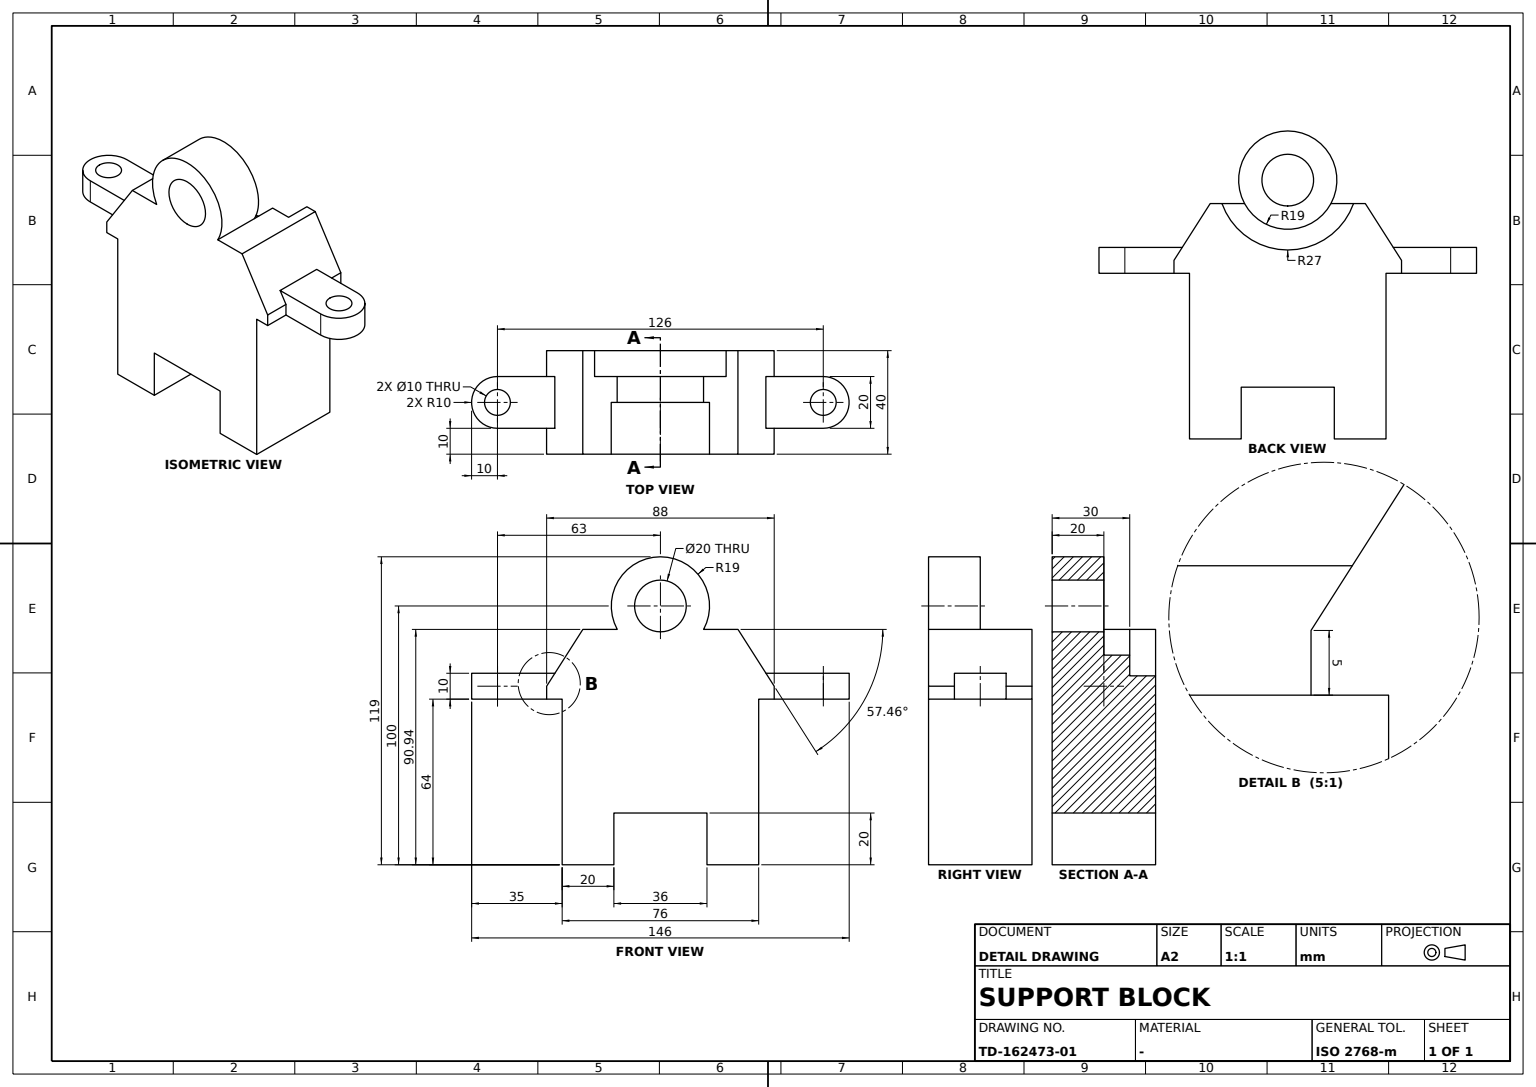
CATIA V5 part; units mm, degrees
sketch "Sketch1" plane through (0, 0, 0) normal (0, 1, 0) x (-1, 0, 0)
  point P0 (-38, 0)
  line L0 (-38, 0) -> (-18, 0)
  line L1 (38, 0) -> (38, 64)
  line L2 (-38, 64) -> (-38, 0)
  line L3 (-38, 64) -> (-44, 64)
  line L4 (-44, 64) -> (-44, 69)
  line L5 (44, 69) -> (44, 64)
  line L6 (44, 64) -> (38, 64)
  line L7 (-18, 0) -> (-18, 20)
  line L8 (-18, 20) -> (18, 20)
  line L9 (18, 20) -> (18, 0)
  point P1 (18, 0)
  line L10 (18, 0) -> (38, 0)
  arc A0 (-25.4361, 90.9444) -> (25.4361, 90.9444) centre (0, 100) ccw
  point P2 (0, 100)
  line L11 (-44, 69) -> (-30, 90.9444)
  point P3 (-30, 90.9444)
  line L12 (44, 69) -> (30, 90.9444)
  point P4 (30, 90.9444)
  line L13 (-30, 90.9444) -> (-25.4361, 90.9444)
  line L14 (25.4361, 90.9444) -> (30, 90.9444)
  dimension "length L1" = 64
  dimension "length L2" = 64
  dimension "distance L2 L1" = 76
  dimension "length L8" = 36
  dimension "length L9" = 20
  dimension "length L5" = 5
  dimension "length L4" = 5
  dimension "distance L4 L5" = 88
  dimension "radius A0" = 27
  dimension "distance P2 L6" = 36
  dimension "distance P2 y axis" = 0
  dimension "distance P3 P4" = 60
  constraint coincidence P0 x-axis
  constraint coincidence P1 L0
  constraint coincidence L0 L10
  constraint horizontal L0 x-axis
  constraint horizontal L3 x-axis
  constraint horizontal L6 x-axis
  constraint horizontal L8 x-axis
  constraint horizontal L10 x-axis
  constraint horizontal L13 x-axis
  constraint horizontal L14 x-axis
  constraint vertical L1 y-axis
  constraint vertical L2 y-axis
  constraint vertical L4 y-axis
  constraint vertical L5 y-axis
  constraint vertical L7 y-axis
  constraint vertical L9 y-axis
  constraint symmetry L2 L1 y-axis
  constraint symmetry L4 L5 y-axis
  constraint symmetry L7 L9 y-axis
  constraint symmetry P3 P4 y-axis
extrude "Pad1" add sketch "Sketch1" along normal mid plane 40
sketch "Sketch2" plane through (0, -20, 0) normal (0, -1, 0) x (1, 0, 0)
  arc A0 (-25.4361, 90.9444) -> (25.4361, 90.9444) centre (0, 100) ccw
  arc A1 (-16.7032, 90.9444) -> (16.7032, 90.9444) centre (0, 100) ccw
  point P0 (0, 100)
  line L0 (-25.4361, 90.9444) -> (-16.7032, 90.9444)
  point P1 (16.7032, 90.9444)
  line L1 (16.7032, 90.9444) -> (25.4361, 90.9444)
  point P2 (11.4413, 84.831)
  dimension "radius A1" = 19
  constraint coincidence P0 y-axis
  constraint coincidence L0 P1
  constraint coincidence L0 L1
  constraint coincidence P2 A1
  constraint concentricity A1 A0
  constraint horizontal L0 x-axis
  constraint horizontal L1 x-axis
extrude "Pad2" add sketch "Sketch2" against normal blind 30
sketch "Sketch3" plane through (0, -20, 0) normal (0, -1, 0) x (1, 0, 0)
  circle A0 centre (0, 100) radius 19
  point P0 (0, 100)
  arc A1 (-16.7032, 90.9444) -> (16.7032, 90.9444) centre (0, 100) ccw construction
  arc A2 (-16.7032, 90.9444) -> (16.7032, 90.9444) centre (0, 100) ccw construction
  circle A3 centre (0, 100) radius 10
  dimension "radius A3" = 10
  constraint coincidence P0 y-axis
  constraint coincidence A0 A2
  constraint concentricity A0 A1
extrude "Pad3" add sketch "Sketch3" against normal blind 20
sketch "Sketch4" plane through (0, 0, 64) normal (0, 0, -1) x (1, 0, 0)
  line L0 (33, 10) -> (63, 10)
  line L1 (63, 10) -> (63, -10) construction
  line L2 (63, -10) -> (33, -10)
  line L3 (33, -10) -> (33, 10)
  arc A0 (63, -10) -> (63, 10) centre (63, 0) ccw
  point P0 (63, 0)
  circle A1 centre (63, 0) radius 5
  dimension "distance y axis L1" = 63
  dimension "length L1" = 20
  dimension "length L2" = 30
  dimension "radius A1" = 5
  constraint horizontal L0 x-axis
  constraint horizontal L2 x-axis
  constraint vertical L1 y-axis
  constraint vertical L3 y-axis
  constraint symmetry L2 L0 x-axis
  constraint midpoint P0 L1
  constraint tangency A0 L0
extrude "Pad4" add sketch "Sketch4" against normal blind 10
mirror "Mirror1" about plane through (0, 0, 0) normal (1, 0, 0) of "Pad4"
properties part number "20"
